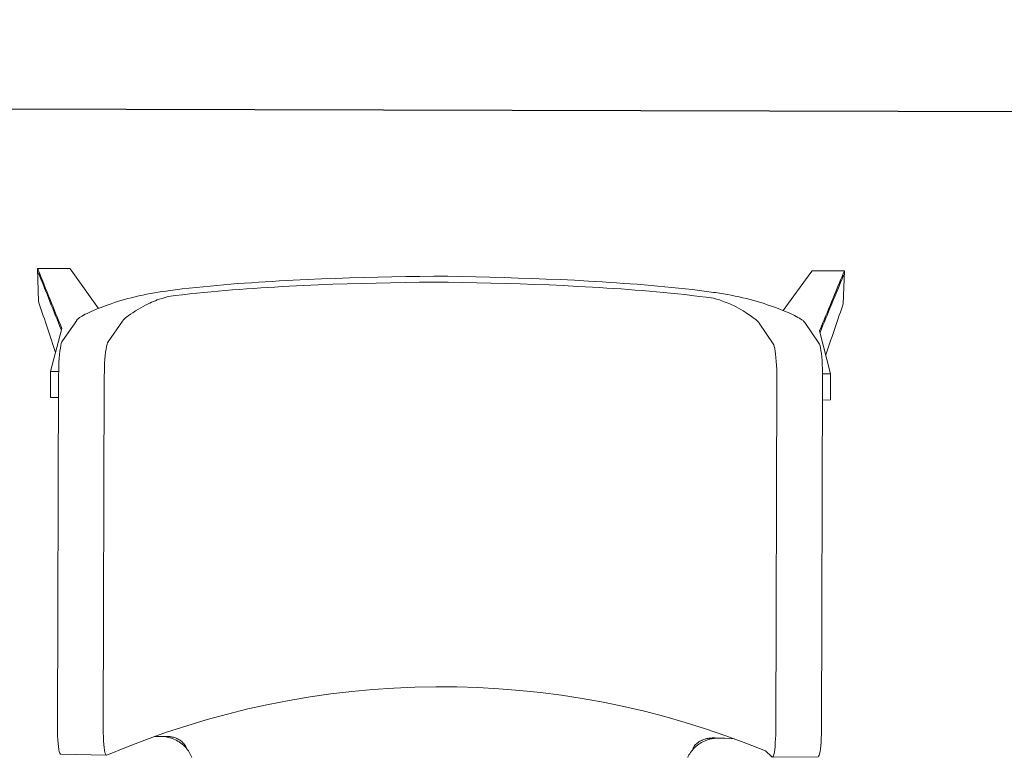
# Model space of a CAD drawing. Units: inches. Extents: x -466983 to 1020, y 324 to 318697.
# Tile 34 of 97: x 847.81 to 867.6, y 741.85 to 756.67. Entities that reach past the tile are written whole.
import ezdxf

# ---------------------------------------------------------------- set-up
doc = ezdxf.new("R2010")
doc.units = ezdxf.units.IN
doc.header["$MEASUREMENT"] = 0
for name, color, linetype, lineweight in [('A-ANNO-DIMS', 2, 'Continuous', 18), ('A-FLOR-PATT', 252, 'Continuous', 13), ('A-FURN', 8, 'Continuous', 18)]:
    doc.layers.add(name, color=color, linetype=linetype, lineweight=lineweight)
doc.layers.add('Office Desk', color=30, linetype='Continuous', true_color=0xeb7500)
doc.styles.get("Standard").update_dxf_attribs({"font": 'arial.ttf'})
doc.dimstyles.get("Standard").update_dxf_attribs({"dimtxt": 6, "dimasz": 4, "dimexe": 3, "dimexo": 3, "dimgap": 0.09, "dimtad": 0, "dimtih": 1, "dimtoh": 1, "dimdec": 1, "dimzin": 0, "dimdsep": 46, "dimlunit": 3, "dimtxsty": 'Standard', "dimcen": 0.09, "dimadec": 0, "dimazin": 0, "dimtfac": 1, "dimtdec": 1, "dimtofl": 0, "dimtmove": 0, "dimatfit": 3, "dimfxl": 1, "dimtolj": 1, "dimtzin": 0, "dimarcsym": 0})

# ---------------------------------------------------------------- blocks, each defined once
blk = doc.blocks.new('Offce Table')
at = {"layer": 'Office Desk'}
blk.add_line((2575.658, 950.355, -0.016), (2635.658, 950.194, -0.016), dxfattribs=at)
blk = doc.blocks.new('Office Chairs')
at = {"ltscale": 60}
for p, q in [((2504.9, 1432.5), (2505.9, 1397.9)), ((2504.9, 1432.5), (2505.7, 1430.6)), ((2504.9, 1432.5), (2538.6, 1432.5)), ((2540, 1430.6), (2538.6, 1432.5)), ((2568.5, 1390.6), (2540, 1430.6)), ((2816.7, 1422.1), (2831.5, 1422.6)), ((2831.5, 1422.6), (2846.2, 1423)), ((2846.2, 1423), (2860.9, 1423.4)), ((2860.9, 1423.4), (2875.7, 1423.7)), ((2875.7, 1423.7), (2890.5, 1424)), ((2890.5, 1424), (2905.1, 1424.2)), ((2905.1, 1424.2), (2919.7, 1424.3)), ((2919.7, 1424.3), (2927.1, 1424.3)), ((2934.4, 1424.3), (2927.1, 1424.3)), ((2949, 1424), (2934.4, 1424.3)), ((2963.6, 1423.8), (2949, 1424)), ((2978.4, 1423.4), (2963.6, 1423.8)), ((2993.2, 1423), (2978.4, 1423.4)), ((3007.9, 1422.5), (2993.2, 1423)), ((3022.6, 1422), (3007.9, 1422.5)), ((3285.5, 1388.4), (3314.3, 1428.2)), ((3314.3, 1428.2), (3315.7, 1430.1)), ((3349.4, 1430), (3315.7, 1430.1)), ((3349.4, 1430), (3348.2, 1395.3)), ((3349.4, 1430), (3348.6, 1428)), ((2663.5, 1411.9), (2670.8, 1412.7)), ((2670.8, 1412.7), (2678.1, 1413.4)), ((2678.1, 1413.4), (2685.4, 1414.1)), ((2685.4, 1414.1), (2692.6, 1414.8)), ((2692.6, 1414.8), (2699.8, 1415.4)), ((2699.8, 1415.4), (2707.1, 1416)), ((2707.1, 1416), (2714.3, 1416.6)), ((2714.3, 1416.6), (2721.5, 1417.1)), ((2721.5, 1417.1), (2728.7, 1417.6)), ((2728.7, 1417.6), (2736, 1418.1)), ((2731, 1411.6), (2738.4, 1412.1)), ((2736, 1418.1), (2743.2, 1418.6)), ((2738.4, 1412.1), (2745.9, 1412.6)), ((2743.2, 1418.6), (2750.5, 1419)), ((2745.9, 1412.6), (2753.4, 1413)), ((2750.5, 1419), (2757.8, 1419.4)), ((2753.4, 1413), (2760.9, 1413.5)), ((2757.8, 1419.4), (2772.5, 1420.2)), ((2760.9, 1413.5), (2768.4, 1413.9)), ((2768.4, 1413.9), (2783.5, 1414.6)), ((2772.5, 1420.2), (2787.2, 1420.9)), ((2783.5, 1414.6), (2798.6, 1415.3)), ((2787.2, 1420.9), (2802, 1421.5)), ((2798.6, 1415.3), (2813.8, 1415.9)), ((2802, 1421.5), (2816.7, 1422.1)), ((2813.8, 1415.9), (2828.9, 1416.4)), ((2828.9, 1416.4), (2844, 1416.8)), ((2844, 1416.8), (2859.2, 1417.2)), ((2859.2, 1417.2), (2874.3, 1417.6)), ((2874.3, 1417.6), (2889.5, 1417.8)), ((2889.5, 1417.8), (2904.5, 1418)), ((2904.5, 1418), (2919.5, 1418.2)), ((2919.5, 1418.2), (2927, 1418.2)), ((2934.5, 1418.1), (2927, 1418.2)), ((2949.6, 1417.9), (2934.5, 1418.1)), ((2964.6, 1417.6), (2949.6, 1417.9)), ((2979.7, 1417.2), (2964.6, 1417.6)), ((2994.9, 1416.8), (2979.7, 1417.2)), ((3010, 1416.3), (2994.9, 1416.8)), ((3025.1, 1415.8), (3010, 1416.3)), ((3037.4, 1421.4), (3022.6, 1422)), ((3040.3, 1415.2), (3025.1, 1415.8)), ((3052.1, 1420.8), (3037.4, 1421.4)), ((3055.4, 1414.5), (3040.3, 1415.2)), ((3066.9, 1420.1), (3052.1, 1420.8)), ((3070.5, 1413.7), (3055.4, 1414.5)), ((3081.6, 1419.3), (3066.9, 1420.1)), ((3085.6, 1412.9), (3070.5, 1413.7)), ((3096.3, 1418.4), (3081.6, 1419.3)), ((3093.2, 1412.4), (3085.6, 1412.9)), ((3100.7, 1412), (3093.2, 1412.4)), ((3103.6, 1417.9), (3096.3, 1418.4)), ((3110.9, 1417.4), (3103.6, 1417.9)), ((3118.1, 1416.9), (3110.9, 1417.4)), ((3125.3, 1416.4), (3118.1, 1416.9)), ((3132.6, 1415.9), (3125.3, 1416.4)), ((3139.8, 1415.3), (3132.6, 1415.9)), ((3147, 1414.7), (3139.8, 1415.3)), ((3154.2, 1414), (3147, 1414.7)), ((3161.4, 1413.4), (3154.2, 1414)), ((3168.7, 1412.7), (3161.4, 1413.4)), ((3175.9, 1411.9), (3168.7, 1412.7)), ((2599.4, 1401), (2603.2, 1401.9)), ((2603.2, 1401.9), (2607, 1402.9)), ((2607, 1402.9), (2610.9, 1403.8)), ((2610.9, 1403.8), (2614.9, 1404.7)), ((2614.9, 1404.7), (2618.9, 1405.5)), ((2618.9, 1405.5), (2623, 1406.3)), ((2623, 1406.3), (2627.1, 1407)), ((2627.1, 1407), (2631.2, 1407.7)), ((2631.2, 1407.7), (2635.3, 1408.3)), ((2635.3, 1408.3), (2639.5, 1408.9)), ((2635.3, 1401.2), (2638.4, 1402.2)), ((2638.4, 1402.2), (2641.6, 1403.1)), ((2639.5, 1408.9), (2641.6, 1409.2)), ((2641.6, 1409.2), (2648.9, 1410.2)), ((2641.6, 1403.1), (2649.1, 1404.1)), ((2648.9, 1410.2), (2656.2, 1411.1)), ((2649.1, 1404.1), (2656.6, 1405)), ((2656.2, 1411.1), (2663.5, 1411.9)), ((2656.6, 1405), (2664.1, 1405.8)), ((2664.1, 1405.8), (2671.6, 1406.6)), ((2671.6, 1406.6), (2679, 1407.4)), ((2679, 1407.4), (2686.5, 1408.1)), ((2686.5, 1408.1), (2693.9, 1408.8)), ((2693.9, 1408.8), (2701.3, 1409.4)), ((2701.3, 1409.4), (2708.8, 1410)), ((2708.8, 1410), (2716.2, 1410.6)), ((2716.2, 1410.6), (2723.6, 1411.1)), ((2723.6, 1411.1), (2731, 1411.6)), ((3108.1, 1411.5), (3100.7, 1412)), ((3115.6, 1411), (3108.1, 1411.5)), ((3123, 1410.4), (3115.6, 1411)), ((3130.4, 1409.9), (3123, 1410.4)), ((3137.9, 1409.3), (3130.4, 1409.9)), ((3145.3, 1408.7), (3137.9, 1409.3)), ((3152.7, 1408), (3145.3, 1408.7)), ((3160.1, 1407.4), (3152.7, 1408)), ((3167.5, 1406.6), (3160.1, 1407.4)), ((3174.9, 1405.9), (3167.5, 1406.6)), ((3182.4, 1405.1), (3174.9, 1405.9)), ((3183.2, 1411.1), (3175.9, 1411.9)), ((3189.9, 1404.2), (3182.4, 1405.1)), ((3190.5, 1410.3), (3183.2, 1411.1)), ((3197.4, 1403.3), (3189.9, 1404.2)), ((3197.8, 1409.4), (3190.5, 1410.3)), ((3204.9, 1402.4), (3197.4, 1403.3)), ((3205.1, 1408.5), (3197.8, 1409.4)), ((3212.4, 1401.3), (3204.9, 1402.4)), ((3212.4, 1407.5), (3205.1, 1408.5)), ((3214.5, 1407.2), (3212.4, 1407.5)), ((3218.7, 1406.6), (3214.5, 1407.2)), ((3222.8, 1405.9), (3218.7, 1406.6)), ((3226.9, 1405.2), (3222.8, 1405.9)), ((3231, 1404.4), (3226.9, 1405.2)), ((3235.1, 1403.6), (3231, 1404.4)), ((3239.1, 1402.8), (3235.1, 1403.6)), ((3243, 1401.9), (3239.1, 1402.8)), ((3246.9, 1400.9), (3243, 1401.9)), ((2506.6, 1395.5), (2505.9, 1397.9)), ((2567.2, 1390.1), (2571.3, 1391.7)), ((2571.3, 1391.7), (2575.7, 1393.4)), ((2575.7, 1393.4), (2578.8, 1394.5)), ((2578.8, 1394.5), (2582, 1395.6)), ((2582, 1395.6), (2585.3, 1396.7)), ((2585.3, 1396.7), (2588.7, 1397.8)), ((2588.7, 1397.8), (2592.2, 1398.9)), ((2592.2, 1398.9), (2595.8, 1399.9)), ((2595.8, 1399.9), (2599.4, 1401)), ((2612.8, 1391.3), (2615.3, 1392.7)), ((2615.3, 1392.7), (2617.9, 1394.1)), ((2617.9, 1394.1), (2620.6, 1395.4)), ((2620.6, 1395.4), (2622.4, 1396.3)), ((2622.4, 1396.3), (2624.3, 1397.1)), ((2624.3, 1397.1), (2626.3, 1397.9)), ((2626.3, 1397.9), (2628.2, 1398.7)), ((2628.2, 1398.7), (2630.2, 1399.5)), ((2630.2, 1399.5), (2632.2, 1400.2)), ((2632.2, 1400.2), (2635.3, 1401.2)), ((3215.5, 1400.4), (3212.4, 1401.3)), ((3218.6, 1399.5), (3215.5, 1400.4)), ((3221.7, 1398.4), (3218.6, 1399.5)), ((3223.7, 1397.7), (3221.7, 1398.4)), ((3225.7, 1396.9), (3223.7, 1397.7)), ((3227.7, 1396.1), (3225.7, 1396.9)), ((3229.6, 1395.3), (3227.7, 1396.1)), ((3231.5, 1394.4), (3229.6, 1395.3)), ((3233.3, 1393.6), (3231.5, 1394.4)), ((3236, 1392.2), (3233.3, 1393.6)), ((3238.6, 1390.8), (3236, 1392.2)), ((3250.8, 1400), (3246.9, 1400.9)), ((3254.5, 1399), (3250.8, 1400)), ((3258.2, 1397.9), (3254.5, 1399)), ((3261.8, 1396.8), (3258.2, 1397.9)), ((3265.3, 1395.7), (3261.8, 1396.8)), ((3268.7, 1394.6), (3265.3, 1395.7)), ((3272, 1393.5), (3268.7, 1394.6)), ((3275.1, 1392.4), (3272, 1393.5)), ((3278.2, 1391.2), (3275.1, 1392.4)), ((3347.4, 1393), (3348.2, 1395.3)), ((2548.8, 1381), (2549.4, 1381.4)), ((2549.4, 1381.4), (2550, 1381.8)), ((2550, 1381.8), (2551.4, 1382.7)), ((2551.4, 1382.7), (2553, 1383.6)), ((2553, 1383.6), (2554.8, 1384.5)), ((2554.8, 1384.5), (2556.7, 1385.5)), ((2556.7, 1385.5), (2558.8, 1386.4)), ((2558.8, 1386.4), (2561, 1387.4)), ((2561, 1387.4), (2563.3, 1388.5)), ((2563.3, 1388.5), (2567.2, 1390.1)), ((2597, 1380.8), (2598.3, 1381.8)), ((2598.3, 1381.8), (2599.8, 1382.9)), ((2599.8, 1382.9), (2602.1, 1384.5)), ((2602.1, 1384.5), (2604.6, 1386.2)), ((2604.6, 1386.2), (2607.4, 1388)), ((2607.4, 1388), (2610.4, 1389.9)), ((2610.4, 1389.9), (2612.8, 1391.3)), ((3241.1, 1389.4), (3238.6, 1390.8)), ((3243.5, 1388), (3241.1, 1389.4)), ((3246.5, 1386.1), (3243.5, 1388)), ((3249.2, 1384.3), (3246.5, 1386.1)), ((3251.8, 1382.5), (3249.2, 1384.3)), ((3254, 1380.9), (3251.8, 1382.5)), ((3282.6, 1389.5), (3278.2, 1391.2)), ((3286.7, 1387.9), (3282.6, 1389.5)), ((3290.5, 1386.3), (3286.7, 1387.9)), ((3292.9, 1385.2), (3290.5, 1386.3)), ((3295.1, 1384.2), (3292.9, 1385.2)), ((3297.2, 1383.2), (3295.1, 1384.2)), ((3299.1, 1382.3), (3297.2, 1383.2)), ((3300.8, 1381.3), (3299.1, 1382.3)), ((3302.4, 1380.4), (3300.8, 1381.3)), ((2530.8, 1356.8), (2545.8, 1378.2)), ((2545.8, 1378.2), (2546.1, 1378.6)), ((2546.1, 1378.6), (2546.4, 1379)), ((2546.4, 1379), (2546.8, 1379.3)), ((2546.8, 1379.3), (2547.2, 1379.7)), ((2547.2, 1379.7), (2547.7, 1380.2)), ((2547.7, 1380.2), (2548.2, 1380.6)), ((2548.2, 1380.6), (2548.8, 1381)), ((2578.7, 1355.8), (2593.6, 1377.3)), ((2593.6, 1377.3), (2594, 1377.8)), ((2594, 1377.8), (2594.4, 1378.3)), ((2594.4, 1378.3), (2594.9, 1378.9)), ((2594.9, 1378.9), (2595.5, 1379.5)), ((2595.5, 1379.5), (2596.2, 1380.1)), ((2596.2, 1380.1), (2597, 1380.8)), ((3255.5, 1379.8), (3254, 1380.9)), ((3256.9, 1378.8), (3255.5, 1379.8)), ((3257.6, 1378.1), (3256.9, 1378.8)), ((3258.3, 1377.5), (3257.6, 1378.1)), ((3258.9, 1376.9), (3258.3, 1377.5)), ((3259.4, 1376.3), (3258.9, 1376.9)), ((3259.8, 1375.8), (3259.4, 1376.3)), ((3260.2, 1375.2), (3259.8, 1375.8)), ((3275, 1353.7), (3260.2, 1375.2)), ((3303.8, 1379.5), (3302.4, 1380.4)), ((3304.4, 1379.1), (3303.8, 1379.5)), ((3305, 1378.7), (3304.4, 1379.1)), ((3305.6, 1378.3), (3305, 1378.7)), ((3306.1, 1377.9), (3305.6, 1378.3)), ((3306.6, 1377.4), (3306.1, 1377.9)), ((3307, 1377), (3306.6, 1377.4)), ((3307.4, 1376.6), (3307, 1377)), ((3307.7, 1376.3), (3307.4, 1376.6)), ((3308, 1375.9), (3307.7, 1376.3)), ((3322.8, 1354.4), (3308, 1375.9)), ((2518.5, 1324.7), (2530.3, 1369.5)), ((3334.9, 1322.2), (3323.5, 1367.1)), ((2529.2, 1351.8), (2528.7, 1349)), ((2529.7, 1354), (2529.2, 1351.8)), ((2530.3, 1355.7), (2529.7, 1354)), ((2530.8, 1356.8), (2530.3, 1355.7)), ((2577.1, 1350.8), (2576.6, 1348.1)), ((2577.6, 1353.1), (2577.1, 1350.8)), ((2578.1, 1354.7), (2577.6, 1353.1)), ((2578.7, 1355.8), (2578.1, 1354.7)), ((3275.5, 1352.6), (3275, 1353.7)), ((3276, 1350.9), (3275.5, 1352.6)), ((3276.5, 1348.7), (3276, 1350.9)), ((3323.3, 1353.3), (3322.8, 1354.4)), ((3323.9, 1351.6), (3323.3, 1353.3)), ((3324.4, 1349.3), (3323.9, 1351.6)), ((2527.9, 1342.3), (2527.6, 1338.4)), ((2528.3, 1345.9), (2527.9, 1342.3)), ((2528.7, 1349), (2528.3, 1345.9)), ((2575.7, 1341.4), (2575.4, 1337.5)), ((2576.1, 1344.9), (2575.7, 1341.4)), ((2576.6, 1348.1), (2576.1, 1344.9)), ((3277, 1346), (3276.5, 1348.7)), ((3277.4, 1342.8), (3277, 1346)), ((3277.8, 1339.2), (3277.4, 1342.8)), ((3324.9, 1346.6), (3324.4, 1349.3)), ((3325.3, 1343.4), (3324.9, 1346.6)), ((3325.7, 1339.9), (3325.3, 1343.4)), ((3326, 1336), (3325.7, 1339.9)), ((2527.1, 1329.9), (2527, 1325.5)), ((2527.3, 1334.3), (2527.1, 1329.9)), ((2527.6, 1338.4), (2527.3, 1334.3)), ((2575.1, 1333.3), (2574.9, 1329)), ((2575.4, 1337.5), (2575.1, 1333.3)), ((3278.1, 1335.3), (3277.8, 1339.2)), ((3278.4, 1331.2), (3278.1, 1335.3)), ((3278.6, 1326.9), (3278.4, 1331.2)), ((3326.2, 1331.8), (3326, 1336)), ((3326.4, 1327.5), (3326.2, 1331.8)), ((2518.5, 1322.2), (2518.5, 1324.7)), ((2518.5, 1324.7), (2521.7, 1324.7)), ((2518.5, 1297.3), (2518.5, 1322.2)), ((2521.7, 1324.7), (2526.9, 1324.6)), ((2525.8, 952.2), (2526.9, 1321.1)), ((2527, 1325.5), (2526.9, 1321.1)), ((2573.6, 951.2), (2574.7, 1320.2)), ((2574.8, 1324.6), (2574.7, 1320.2)), ((2574.9, 1329), (2574.8, 1324.6)), ((3278.7, 1322.5), (3278.6, 1326.9)), ((3278.7, 1318.1), (3278.7, 1322.5)), ((3326.5, 1323.1), (3326.4, 1327.5)), ((3326.5, 1318.7), (3326.5, 1323.1)), ((3331.7, 1322.2), (3326.5, 1322.2)), ((3334.9, 1322.2), (3331.7, 1322.2)), ((3334.8, 1294.9), (3334.9, 1319.7)), ((3334.9, 1319.7), (3334.9, 1322.2)), ((3277.6, 949.1), (3278.7, 1318.1)), ((3325.4, 949.7), (3326.5, 1318.7)), ((2518.5, 1297.3), (2526.8, 1297.3)), ((3334.8, 1294.9), (3326.4, 1294.8)), ((2525.8, 952.2), (2525.8, 947.6)), ((2573.6, 951.2), (2573.6, 946.7)), ((3277.5, 944.6), (3277.6, 949.1)), ((3325.3, 945.2), (3325.4, 949.7)), ((2525.8, 947.6), (2525.9, 943.3)), ((2525.9, 943.3), (2526.1, 939.2)), ((2526.1, 939.2), (2526.4, 935.4)), ((2573.6, 946.7), (2573.8, 942.3)), ((2573.8, 942.3), (2574, 938.2)), ((2574, 938.2), (2574.2, 934.5)), ((2633.9, 942.8), (2627, 942.7)), ((2634.8, 942.8), (2633.9, 942.8)), ((2635.6, 942.8), (2634.8, 942.8)), ((2636.5, 942.8), (2635.6, 942.8)), ((2637.3, 942.7), (2636.5, 942.8)), ((2638.2, 942.6), (2637.3, 942.7)), ((2639, 942.5), (2638.2, 942.6)), ((2639.9, 942.3), (2639, 942.5)), ((2640.7, 942.2), (2639.9, 942.3)), ((2641.5, 942.8), (2640.1, 942.9)), ((2641.6, 942), (2640.7, 942.2)), ((2643, 942.7), (2641.5, 942.8)), ((2642.4, 941.7), (2641.6, 942)), ((2643.3, 941.5), (2642.4, 941.7)), ((2643.7, 942.6), (2643, 942.7)), ((2644.1, 941.3), (2643.3, 941.5)), ((2644.4, 942.5), (2643.7, 942.6)), ((2645, 941), (2644.1, 941.3)), ((2645.1, 942.4), (2644.4, 942.5)), ((2645.8, 940.7), (2645, 941)), ((2645.8, 942.2), (2645.1, 942.4)), ((2646.4, 942.1), (2645.8, 942.2)), ((2646.7, 940.3), (2645.8, 940.7)), ((2647.1, 941.9), (2646.4, 942.1)), ((2647.5, 940), (2646.7, 940.3)), ((2647.8, 941.6), (2647.1, 941.9)), ((2649.1, 939.3), (2647.5, 940)), ((2650.7, 938.4), (2649.1, 939.3)), ((2651.1, 940.3), (2650.5, 940.5)), ((2651.5, 938), (2650.7, 938.4)), ((2652.1, 939.9), (2651.1, 940.3)), ((2652.3, 937.5), (2651.5, 938)), ((2653.1, 939.4), (2652.1, 939.9)), ((2654, 938.8), (2653.1, 939.4)), ((2655, 938.2), (2654, 938.8)), ((2655.8, 937.5), (2655, 938.2)), ((3198.1, 937.7), (3199.1, 938.2)), ((3199.1, 938.2), (3200.1, 938.7)), ((3200.1, 938.7), (3200.6, 938.9)), ((3202, 937.6), (3203.7, 938.3)), ((3203.4, 939.9), (3204.1, 940.2)), ((3203.7, 938.3), (3204.5, 938.6)), ((3204.1, 940.2), (3204.7, 940.4)), ((3204.5, 938.6), (3205.3, 939)), ((3204.7, 940.4), (3205.4, 940.5)), ((3205.3, 939), (3206.2, 939.3)), ((3205.4, 940.5), (3206.1, 940.7)), ((3206.1, 940.7), (3206.8, 940.8)), ((3206.2, 939.3), (3207, 939.5)), ((3206.8, 940.8), (3207.5, 940.9)), ((3207, 939.5), (3207.9, 939.8)), ((3207.5, 940.9), (3208.2, 941)), ((3207.9, 939.8), (3208.7, 940)), ((3208.2, 941), (3209.6, 941.1)), ((3208.7, 940), (3209.6, 940.2)), ((3209.6, 941.1), (3211.1, 941.1)), ((3209.6, 940.2), (3210.4, 940.4)), ((3210.4, 940.4), (3211.3, 940.6)), ((3211.3, 940.6), (3212.2, 940.7)), ((3212.2, 940.7), (3213, 940.8)), ((3213, 940.8), (3213.9, 940.9)), ((3213.9, 940.9), (3214.7, 941)), ((3214.7, 941), (3215.6, 941.1)), ((3215.6, 941.1), (3216.4, 941.1)), ((3216.4, 941.1), (3217.3, 941.1)), ((3224.2, 940.9), (3217.3, 941.1)), ((3230.8, 940.5), (3224.2, 940.9)), ((3234.4, 940.3), (3230.8, 940.5)), ((3277.1, 936.1), (3277.4, 940.2)), ((3277.4, 940.2), (3277.5, 944.6)), ((3325, 936.7), (3325.2, 940.8)), ((3325.2, 940.8), (3325.3, 945.2)), ((2526.4, 935.4), (2526.7, 932.1)), ((2526.7, 932.1), (2527.2, 929.3)), ((2527.2, 929.3), (2527.6, 927)), ((2574.2, 934.5), (2574.6, 931.2)), ((2574.6, 931.2), (2575, 928.4)), ((2575, 928.4), (2575.4, 926.1)), ((2653, 937.1), (2652.3, 937.5)), ((2653.8, 936.6), (2653, 937.1)), ((2654.5, 936.1), (2653.8, 936.6)), ((2655.2, 935.5), (2654.5, 936.1)), ((2655.9, 935), (2655.2, 935.5)), ((2656.7, 936.7), (2655.8, 937.5)), ((2656.6, 934.5), (2655.9, 935)), ((2657.3, 933.9), (2656.6, 934.5)), ((2657.4, 935.9), (2656.7, 936.7)), ((2657.9, 933.3), (2657.3, 933.9)), ((2658.2, 935.1), (2657.4, 935.9)), ((2658.5, 932.7), (2657.9, 933.3)), ((2658.8, 934.2), (2658.2, 935.1)), ((2659.1, 932.1), (2658.5, 932.7)), ((2659.4, 933.2), (2658.8, 934.2)), ((2659.7, 931.5), (2659.1, 932.1)), ((2659.9, 932.2), (2659.4, 933.2)), ((2660.3, 930.8), (2659.7, 931.5)), ((2660.4, 931.2), (2659.9, 932.2)), ((2660.8, 930.2), (2660.3, 930.8)), ((2660.8, 930.2), (2660.4, 931.2)), ((2660.8, 930.2), (2661.8, 928.9)), ((2661.8, 928.9), (2662.7, 927.6)), ((2662.7, 927.6), (2663.6, 926.3)), ((3190.3, 928.6), (3189.3, 927.3)), ((3190.3, 928.6), (3190.7, 929.6)), ((3190.3, 928.6), (3190.8, 929.2)), ((3190.7, 929.6), (3191.2, 930.6)), ((3190.8, 929.2), (3191.4, 929.9)), ((3191.2, 930.6), (3191.7, 931.6)), ((3191.4, 929.9), (3192, 930.5)), ((3191.7, 931.6), (3192.3, 932.6)), ((3192, 930.5), (3192.6, 931.1)), ((3192.3, 932.6), (3193, 933.5)), ((3192.6, 931.1), (3193.2, 931.7)), ((3193, 933.5), (3193.7, 934.3)), ((3193.2, 931.7), (3193.9, 932.3)), ((3193.7, 934.3), (3194.5, 935.1)), ((3193.9, 932.3), (3194.5, 932.8)), ((3194.5, 935.1), (3195.3, 935.9)), ((3194.5, 932.8), (3195.2, 933.4)), ((3195.2, 933.4), (3195.9, 933.9)), ((3195.3, 935.9), (3196.2, 936.5)), ((3195.9, 933.9), (3196.6, 934.4)), ((3196.2, 936.5), (3197.1, 937.2)), ((3196.6, 934.4), (3197.4, 934.9)), ((3197.1, 937.2), (3198.1, 937.7)), ((3197.4, 934.9), (3198.1, 935.4)), ((3198.1, 935.4), (3198.9, 935.9)), ((3198.9, 935.9), (3199.6, 936.3)), ((3199.6, 936.3), (3200.4, 936.8)), ((3200.4, 936.8), (3202, 937.6)), ((3267, 927.6), (3273.4, 921.3)), ((3276.1, 926.3), (3276.5, 929.1)), ((3276.5, 929.1), (3276.9, 932.4)), ((3276.9, 932.4), (3277.1, 936.1)), ((3323.9, 926.9), (3324.3, 929.7)), ((3324.3, 929.7), (3324.7, 933)), ((3324.7, 933), (3325, 936.7)), ((2527.6, 927), (2528.1, 925.4)), ((2528.1, 925.4), (2528.7, 924.4)), ((2528.7, 924.4), (2529.2, 924.1)), ((2529.2, 924.1), (2577.1, 923.1)), ((2575.4, 926.1), (2576, 924.5)), ((2576, 924.5), (2576.5, 923.5)), ((2576.5, 923.5), (2577.1, 923.1)), ((2577.1, 923.1), (2577.1, 923.1)), ((2577.1, 923.1), (2577.2, 923.1)), ((2663.6, 926.3), (2664.3, 925)), ((2664.3, 925), (2665, 923.6)), ((2665, 923.6), (2665.7, 922.3)), ((2665.7, 922.3), (2666.3, 920.9)), ((3186, 922.1), (3185.4, 920.7)), ((3186.7, 923.4), (3186, 922.1)), ((3187.5, 924.7), (3186.7, 923.4)), ((3188.4, 926), (3187.5, 924.7)), ((3189.3, 927.3), (3188.4, 926)), ((3273.4, 921.3), (3273.5, 921.2)), ((3273.5, 921.2), (3273.5, 921.2)), ((3273.5, 921.2), (3273.6, 921.1)), ((3273.6, 921.1), (3273.7, 921.1)), ((3273.7, 921.1), (3273.7, 921.1)), ((3273.7, 921.1), (3273.8, 921)), ((3273.8, 921), (3273.8, 921)), ((3273.8, 921), (3273.9, 921)), ((3273.9, 921), (3321.8, 921.6)), ((3273.9, 921), (3274.5, 921.4)), ((3273.9, 921), (3273.9, 921)), ((3274.5, 921.4), (3275.1, 922.4)), ((3275.1, 922.4), (3275.6, 924)), ((3275.6, 924), (3276.1, 926.3)), ((3321.8, 921.6), (3322.4, 922)), ((3322.4, 922), (3322.9, 923)), ((3322.9, 923), (3323.4, 924.6)), ((3323.4, 924.6), (3323.9, 926.9))]:
    blk.add_line(p, q, dxfattribs=at)
for centre, radius, start, end in [((-145493.7, -58276.8), 159589.4, 21.947005, 21.970624), ((-144608, -57922.2), 158634.4, 21.947319, 21.970637), ((151110, -59414.6), 159797.6, 157.619968, 157.643565), ((150230.4, -59055.2), 158846.4, 157.619943, 157.643251), ((-168189.3, -55680.2), 179985.4, 18.471313, 18.488444), ((173897.2, -56966.9), 180258.5, 161.10973, 161.126868), ((2639.1, 564.4), 378.5, 89.8391, 90.7789), ((2641.9, 923), 19.6, 63.7894, 72.4249), ((3209.2, 921.2), 19.6, 107.2271, 115.8628), ((3209.8, 562.7), 378.5, 88.873, 89.8128)]:
    blk.add_arc(centre, radius, start, end, dxfattribs=at)
blk.add_arc((2927.4, 103.4), 891.4, 67.6085, 113.1294)
blk = doc.blocks.new('Office Desk With Chairs')
blk.add_blockref('Offce Table', (-526.404, 94.584))
at = {"xscale": 0.0191941550942558, "yscale": 0.0191941550942558, "zscale": 0.0191941550942558}
blk.add_blockref('Office Chairs', (2012.509, 1014.21), dxfattribs=at)
blk = doc.blocks.new('*D99')
at = {"layer": 'A-ANNO-DIMS', "color": 0, "lineweight": -2, "transparency": 16777216}
for p, q in [((833.84, 822.679), (820.85, 822.679)), ((823.85, 818.679), (823.85, 782.572)), ((823.85, 740.077), (823.85, 776.184)), ((833.84, 736.077), (820.85, 736.077))]:
    blk.add_line(p, q, dxfattribs=at)
at = {"layer": 'A-ANNO-DIMS', "color": 0, "transparency": 16777216}
for points in [[(823.183, 818.679), (824.517, 818.679), (823.85, 822.679)], [(823.183, 740.077), (824.517, 740.077), (823.85, 736.077)]]:
    blk.add_solid(points, dxfattribs=at)
at = {"layer": 'Defpoints', "color": 0, "transparency": 16777216}
for p in [(823.85, 822.679), (836.84, 822.679), (836.84, 736.077)]:
    blk.add_point(p, dxfattribs=at)
at = {"layer": 'A-ANNO-DIMS', "color": 0, "transparency": 16777216, "insert": (823.85, 779.378), "char_height": 6, "attachment_point": 5}
blk.add_mtext('\\A1;OFFICE DESK 87', dxfattribs=at)

msp = doc.modelspace()

# ---------------------------------------------------------------- hatches: boundary and pattern name
at = {"layer": 'A-FLOR-PATT', "transparency": 33554572}
h = msp.add_hatch(dxfattribs=at)
h.set_pattern_fill('ANSI37', color=256, scale=30)
h.set_pattern_definition([(45, (-1212.4137, -290.035), (-2.6516504, 2.6516504), []), (135, (-1212.4137, -290.035), (-2.6516504, -2.6516504), [])])
h.paths.add_polyline_path([(901.806, 1075.938), (900.614, 1075.938), (900.614, 1065.386), (899.391, 1065.386), (898.091, 1065.386), (892.836, 1058.71, -0.258377), (892.188, 1058.351), (879.985, 1058.351, -0.20177), (879.438, 1058.581), (874.081, 1065.386), (872.781, 1065.386), (871.558, 1065.386), (871.558, 1075.938), (813.806, 1075.938), (813.806, 1044.792), (832.395, 1044.792, -0.394795), (848.66, 1028.536), (848.66, 1009.938), (901.806, 1009.938), (901.806, 1015.938), (901.306, 1015.938), (871.306, 1015.938), (871.306, 1017.25), (871.334, 1017.25, -0.401453), (901.306, 1045.938), (901.806, 1045.938)])
edge = h.paths.add_edge_path(flags=16)
edge.add_line((847.773, 1068.949), (847.773, 1073.709))
edge.add_arc((849.227, 1073.709), 1.454, 90, 180, ccw=False)
edge.add_line((849.227, 1075.163), (864.492, 1075.163))
edge.add_arc((864.492, 1073.709), 1.454, 0, 90, ccw=False)
edge.add_line((865.946, 1073.709), (865.946, 1069.004))
edge.add_arc((832.645, 1068.976), 33.301, -20.6123, 0.0472, ccw=False)
edge.add_ellipse((856.859, 1058.48), major_axis=(0, 10.213), ratio=0.685919, start_angle=100.0088, end_angle=259.9912, ccw=False)
edge.add_arc((881.074, 1068.976), 33.301, 180.0472, 200.6123, ccw=False)
h.paths.add_polyline_path([(853.146, 1066.482), (853.146, 1066.453), (853.146, 1066.453, 0.433107), (852.917, 1066.685), (852.917, 1066.453), (853.146, 1066.453), (853.146, 1066.482), (853.088, 1066.612, 0.697939), (852.7, 1066.453), (852.7, 1066.453), (852.7, 1066.482), (852.917, 1067.001), (852.917, 1066.685, -0.396254)], flags=0)
h.paths.add_polyline_path([(861.019, 1066.482), (861.019, 1066.453), (861.019, 1066.453, 0.416404), (860.802, 1066.685), (860.802, 1066.453), (861.019, 1066.453), (861.019, 1066.482), (860.967, 1066.605, 0.713344), (860.573, 1066.453), (860.573, 1066.453), (860.573, 1066.482), (860.802, 1067.001), (860.802, 1066.685, -0.379973)], flags=0)
edge = h.paths.add_edge_path(flags=0)
edge.add_spline(control_points=[(861.13, 1065.785), (861.466, 1065.248), (861.613, 1065.016), (861.983, 1064.374), (862.192, 1063.944), (862.561, 1063.039), (862.721, 1062.563), (862.987, 1061.578), (863.092, 1061.069), (863.245, 1060.031), (863.293, 1059.503), (863.329, 1058.441), (863.318, 1057.908), (863.237, 1056.852), (863.166, 1056.329), (862.97, 1055.308), (862.843, 1054.81), (862.537, 1053.852), (862.357, 1053.393), (861.951, 1052.525), (861.725, 1052.117), (861.233, 1051.362), (860.967, 1051.016), (860.405, 1050.395), (860.108, 1050.12), (859.494, 1049.646), (859.176, 1049.448), (858.528, 1049.13), (858.197, 1049.011), (857.531, 1048.852), (857.196, 1048.812), (856.525, 1048.812), (856.189, 1048.852), (855.524, 1049.01), (855.193, 1049.129), (854.545, 1049.447), (854.227, 1049.645), (853.612, 1050.118), (853.316, 1050.393), (852.753, 1051.014), (852.487, 1051.36), (851.995, 1052.114), (851.769, 1052.523), (851.363, 1053.39), (851.183, 1053.85), (850.877, 1054.807), (850.75, 1055.305), (850.553, 1056.326), (850.483, 1056.849), (850.401, 1057.905), (850.39, 1058.438), (850.426, 1059.5), (850.473, 1060.028), (850.626, 1061.066), (850.732, 1061.575), (850.997, 1062.561), (851.157, 1063.036), (851.525, 1063.942), (851.734, 1064.371), (852.106, 1065.016), (852.254, 1065.25), (852.608, 1065.733)], knot_values=[3.915332, 3.915332, 3.915332, 3.915332, 4.013468, 4.013468, 4.175532, 4.175532, 4.337596, 4.337596, 4.49966, 4.49966, 4.661724, 4.661724, 4.823788, 4.823788, 4.985852, 4.985852, 5.147916, 5.147916, 5.30998, 5.30998, 5.472044, 5.472044, 5.634109, 5.634109, 5.796173, 5.796173, 5.958237, 5.958237, 6.120301, 6.120301, 6.282365, 6.282365, 6.444429, 6.444429, 6.606493, 6.606493, 6.768557, 6.768557, 6.930621, 6.930621, 7.092685, 7.092685, 7.254749, 7.254749, 7.416813, 7.416813, 7.578878, 7.578878, 7.740942, 7.740942, 7.903006, 7.903006, 8.06507, 8.06507, 8.227134, 8.227134, 8.389198, 8.389198, 8.551262, 8.551262, 8.65037, 8.65037, 8.65037, 8.65037], degree=3, periodic=0)
edge.add_line((852.642, 1065.785), (861.13, 1065.785))
edge = h.paths.add_edge_path(flags=0)
edge.add_ellipse((856.85, 1057.743), major_axis=(0, 7.792), ratio=0.687861, start_angle=0, end_angle=360)
h.paths.add_polyline_path([(848.863, 1069.389), (848.863, 1073.96, -0.414214), (849.954, 1075.051), (863.765, 1075.051, -0.414214), (864.856, 1073.96), (864.856, 1069.389, -0.388936), (864.524, 1069.027, -0.043561), (849.195, 1069.027, -0.388936)], flags=0)
h.paths.add_polyline_path([(853.101, 1068.112, -1), (852.677, 1068.112, -1)], flags=0)
edge = h.paths.add_edge_path(flags=0)
edge.add_ellipse((856.859, 1057.338), major_axis=(0, 2.207), ratio=0.657164, start_angle=0, end_angle=360)
h.paths.add_polyline_path([(861.041, 1068.112, -1), (860.618, 1068.112, -1)], flags=0)
edge = h.paths.add_edge_path()
edge.add_line((573.954, 1057.341), (573.954, 1075.938))
edge.add_line((573.954, 1075.938), (558.731, 1075.938))
edge.add_line((558.731, 1075.938), (558.731, 1065.386))
edge.add_line((558.731, 1065.386), (557.507, 1065.386))
edge.add_line((557.507, 1065.386), (556.207, 1065.386))
edge.add_line((556.207, 1065.386), (550.952, 1058.71))
edge.add_arc((550.304, 1059.116), 0.765, 270, 327.9483, ccw=False)
edge.add_line((550.304, 1058.351), (538.101, 1058.351))
edge.add_arc((538.101, 1059.116), 0.765, 224.3704, 270, ccw=False)
edge.add_line((537.555, 1058.581), (532.198, 1065.386))
edge.add_line((532.198, 1065.386), (530.898, 1065.386))
edge.add_line((530.898, 1065.386), (529.674, 1065.386))
edge.add_line((529.674, 1065.386), (529.674, 1075.938))
edge.add_line((529.674, 1075.938), (520.806, 1075.938))
edge.add_line((520.806, 1075.938), (520.806, 1045.938))
edge.add_line((520.806, 1045.938), (521.306, 1045.938))
edge.add_arc((521.306, 1015.938), 30, 2.5075, 90, ccw=False)
edge.add_line((551.277, 1017.25), (551.306, 1017.25))
edge.add_line((551.306, 1017.25), (551.306, 1015.938))
edge.add_line((551.306, 1015.938), (520.806, 1015.938))
edge.add_line((520.806, 1015.938), (520.806, 1009.938))
edge.add_line((520.806, 1009.938), (559.191, 1010.402))
edge.add_arc((559.191, 1011.856), 1.454, 180, 270, ccw=False)
edge.add_line((557.737, 1011.856), (557.737, 1016.561))
edge.add_arc((591.039, 1016.589), 33.301, 159.3877, 180.0472, ccw=False)
edge.add_ellipse((566.824, 1027.085), major_axis=(0, 10.213), ratio=0.685919, start_angle=280.0088, end_angle=439.9912, ccw=False)
edge.add_arc((542.609, 1016.589), 33.301, 0.0472, 20.6123, ccw=False)
edge.add_line((575.91, 1016.616), (575.91, 1011.856))
edge.add_arc((574.456, 1011.856), 1.454, -90, 0, ccw=False)
edge.add_line((574.456, 1010.402), (608.806, 1009.938))
edge.add_line((608.806, 1009.938), (608.806, 1041.086))
edge.add_line((608.806, 1041.086), (590.218, 1041.086))
edge.add_arc((590.775, 1057.907), 16.831, 181.9277, 268.1032, ccw=False)
edge = h.paths.add_edge_path()
edge.add_ellipse((494.244, 583.62), major_axis=(0, 10.213), ratio=0.685919, start_angle=280.0088, end_angle=439.9912, ccw=False)
edge.add_arc((470.03, 573.124), 33.301, 0.0472, 20.6123, ccw=False)
edge.add_line((503.331, 573.152), (503.331, 568.392))
edge.add_arc((501.877, 568.392), 1.454, -90, 0, ccw=False)
edge.add_line((501.877, 566.938), (539.806, 566.938))
edge.add_line((539.806, 566.938), (539.806, 572.938))
edge.add_line((539.806, 572.938), (539.306, 572.938))
edge.add_line((539.306, 572.938), (509.306, 572.938))
edge.add_line((509.306, 572.938), (509.306, 574.25))
edge.add_line((509.306, 574.25), (509.334, 574.25))
edge.add_arc((539.306, 572.938), 30, 90, 177.4925, ccw=False)
edge.add_line((539.306, 602.938), (539.806, 602.938))
edge.add_line((539.806, 602.938), (539.806, 626.938))
edge.add_line((539.806, 626.938), (531.772, 626.938))
edge.add_line((531.772, 626.938), (531.772, 616.386))
edge.add_line((531.772, 616.386), (530.548, 616.386))
edge.add_line((530.548, 616.386), (529.249, 616.386))
edge.add_line((529.249, 616.386), (523.711, 609.351))
edge.add_line((523.711, 609.351), (510.777, 609.351))
edge.add_line((510.777, 609.351), (505.239, 616.386))
edge.add_line((505.239, 616.386), (503.939, 616.386))
edge.add_line((503.939, 616.386), (502.715, 616.386))
edge.add_line((502.715, 616.386), (502.715, 626.938))
edge.add_line((502.715, 626.938), (481.698, 626.938))
edge.add_line((481.698, 626.938), (481.698, 610.995))
edge.add_arc((467.27, 611.473), 14.436, 271.9277, 358.1032, ccw=False)
edge.add_line((467.756, 597.045), (451.806, 597.045))
edge.add_line((451.806, 597.045), (451.806, 584.404))
edge.add_line((451.806, 584.404), (451.806, 566.938))
edge.add_line((451.806, 566.938), (486.612, 566.938))
edge.add_arc((486.612, 568.392), 1.454, 180, 270, ccw=False)
edge.add_line((485.158, 568.392), (485.158, 573.097))
edge.add_arc((518.459, 573.124), 33.301, 159.3877, 180.0472, ccw=False)
h.paths.add_polyline_path([(836.261, 1020.733), (879.89, 1020.733), (879.89, 1039.39), (836.261, 1039.39)], flags=25)
h.paths.add_polyline_path([(549.985, 1036.749), (593.614, 1036.749), (593.614, 1055.407), (549.985, 1055.407)], flags=24)
h.paths.add_polyline_path([(475.123, 595.596), (518.752, 595.596), (518.752, 614.253), (475.123, 614.253)], flags=24)

# ---------------------------------------------------------------- block references
at = {"layer": 'A-FURN'}
msp.add_blockref('Office Desk With Chairs', (-1212.414, -290.035), dxfattribs=at)

# ---------------------------------------------------------------- dimensions: what is measured, and where the dimension line sits
at = {"layer": 'A-ANNO-DIMS'}
dim = msp.add_linear_dim(base=(823.85, 822.679), p1=(836.84, 736.077), p2=(836.84, 822.679), angle=90, text='OFFICE DESK <>', dimstyle='Standard', override={"dimdec": 0, "dimlfac": 1, "dimrnd": 0, "dimzin": 0, "dimdsep": 46, "dimlunit": 2}, dxfattribs=at)
dim.commit()
dim.dimension.update_dxf_attribs({"geometry": '*D99', "text_midpoint": (823.85, 779.378)})

doc.saveas('drawing.dxf')
